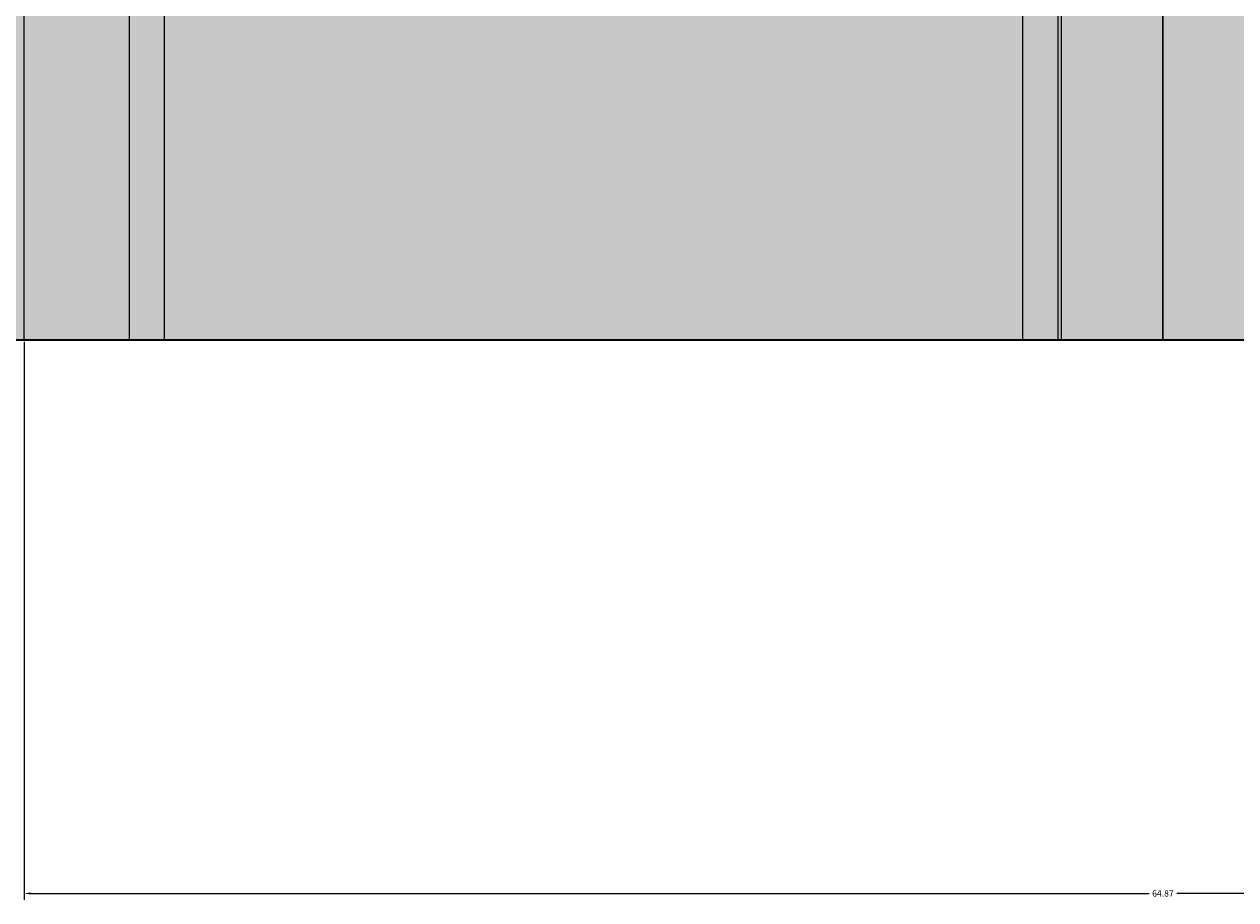
# Model space of a CAD drawing. Units: feet. Extents: x 2695 to 2912, y 795 to 1139.
# Tile 16 of 83: x 2774 to 2808, y 795 to 820. Entities that reach past the tile are written whole.
import ezdxf

# ---------------------------------------------------------------- set-up
doc = ezdxf.new("R2010")
doc.units = ezdxf.units.FT
for name, color, linetype, lineweight in [('A-ANNO-DIMS', 2, 'Continuous', 18), ('A-DOOR', 3, 'Continuous', 25), ('A-DOOR-PATT', 33, 'Continuous', 13), ('A-ELEV', 7, 'Continuous', 35), ('A-ELEV-PATT', 252, 'Continuous', 13)]:
    doc.layers.add(name, color=color, linetype=linetype, lineweight=lineweight)
doc.styles.get("Standard").update_dxf_attribs({"font": 'arial.ttf'})
doc.dimstyles.get("Standard").update_dxf_attribs({"dimtxt": 0.18, "dimasz": 0.18, "dimexe": 0.18, "dimexo": 0.0625, "dimgap": 0.09, "dimtad": 0, "dimtih": 1, "dimtoh": 1, "dimdec": 1, "dimzin": 0, "dimdsep": 46, "dimlunit": 3, "dimtxsty": 'Standard', "dimcen": 0.09, "dimadec": 0, "dimazin": 0, "dimtfac": 1, "dimtdec": 1, "dimtofl": 0, "dimtmove": 0, "dimatfit": 3, "dimfxl": 1, "dimtolj": 1, "dimtzin": 0, "dimarcsym": 0})

# ---------------------------------------------------------------- blocks, each defined once
blk = doc.blocks.new('*D5')
at = {"layer": 'A-ANNO-DIMS', "color": 0, "lineweight": -2, "transparency": 16777216}
for p, q in [((2773.503, 810.868), (2773.503, 794.976)), ((2838.377, 810.868), (2838.377, 794.976)), ((2773.683, 795.156), (2805.546, 795.156)), ((2838.197, 795.156), (2806.334, 795.156))]:
    blk.add_line(p, q, dxfattribs=at)
at = {"layer": 'A-ANNO-DIMS', "color": 0, "transparency": 16777216}
for points in [[(2773.683, 795.186), (2773.683, 795.126), (2773.503, 795.156)], [(2838.197, 795.186), (2838.197, 795.126), (2838.377, 795.156)]]:
    blk.add_solid(points, dxfattribs=at)
at = {"layer": 'Defpoints', "color": 0, "transparency": 16777216}
for p in [(2773.503, 810.931), (2838.377, 810.931), (2838.377, 795.156)]:
    blk.add_point(p, dxfattribs=at)
at = {"layer": 'A-ANNO-DIMS', "color": 0, "transparency": 16777216, "insert": (2805.94, 795.156), "char_height": 0.18, "attachment_point": 5}
blk.add_mtext('\\A1;64.87', dxfattribs=at)
blk = doc.blocks.new('*D13')
at = {"layer": 'A-ANNO-DIMS', "color": 0, "lineweight": -2, "transparency": 16777216}
for p, q in [((2758.214, 874.857), (2911.424, 874.857)), ((2911.244, 874.677), (2911.244, 843.076)), ((2911.244, 811.111), (2911.244, 842.712)), ((2890.699, 810.931), (2911.424, 810.931))]:
    blk.add_line(p, q, dxfattribs=at)
at = {"layer": 'A-ANNO-DIMS', "color": 0, "transparency": 16777216}
for points in [[(2911.214, 874.677), (2911.274, 874.677), (2911.244, 874.857)], [(2911.214, 811.111), (2911.274, 811.111), (2911.244, 810.931)]]:
    blk.add_solid(points, dxfattribs=at)
at = {"layer": 'Defpoints', "color": 0, "transparency": 16777216}
for p in [(2758.151, 874.857), (2911.244, 874.857), (2890.636, 810.931)]:
    blk.add_point(p, dxfattribs=at)
at = {"layer": 'A-ANNO-DIMS', "color": 0, "transparency": 16777216, "insert": (2911.244, 842.894), "char_height": 0.18, "attachment_point": 5}
blk.add_mtext('\\A1;63.93', dxfattribs=at)

msp = doc.modelspace()

# ---------------------------------------------------------------- hatches: boundary and pattern name
at = {"layer": 'A-DOOR-PATT'}
h = msp.add_hatch(color=256, dxfattribs=at)
h.set_gradient(color1=(211, 185, 150), color2=(211, 185, 150))
h.paths.add_polyline_path([(2805.9398, 905.5143), (2773.5029, 905.5143), (2773.5029, 810.9306), (2776.4999, 810.9306), (2776.4999, 902.5174), (2802.9429, 902.5174), (2802.9429, 810.9306), (2805.9398, 810.9306)])
h.paths.add_polyline_path([(2803.9681, 874.1057), (2805.0538, 874.1057), (2805.0538, 846.2857), (2803.9681, 846.2857)], flags=16)
h.paths.add_polyline_path([(2838.3767, 905.5143), (2805.9398, 905.5143), (2805.9398, 810.9306), (2808.9368, 810.9306), (2808.9368, 902.5174), (2835.3798, 902.5174), (2835.3798, 810.9306), (2838.3767, 810.9306)])
h = msp.add_hatch(color=256, dxfattribs=at)
h.set_gradient(color1=(211, 185, 150), color2=(211, 185, 150))
h.paths.add_polyline_path([(2777.5029, 901.5143), (2801.9398, 901.5143), (2801.9398, 810.9306), (2802.9429, 810.9306), (2802.9429, 902.5174), (2776.4999, 902.5174), (2776.4999, 810.9306), (2777.5029, 810.9306)])
h.paths.add_polyline_path([(2809.9398, 901.5143), (2834.3767, 901.5143), (2834.3767, 810.9306), (2835.3798, 810.9306), (2835.3798, 902.5174), (2808.9368, 902.5174), (2808.9368, 810.9306), (2809.9398, 810.9306)])
h = msp.add_hatch(color=256, dxfattribs=at)
h.set_gradient(color1=(173, 221, 247), color2=(173, 221, 247))
h.paths.add_polyline_path([(2801.9398, 901.5143), (2777.5029, 901.5143), (2777.5029, 810.9306), (2801.9398, 810.9306)])
h.paths.add_polyline_path([(2834.3767, 901.5143), (2809.9398, 901.5143), (2809.9398, 810.9306), (2834.3767, 810.9306)])
at = {"layer": 'A-ELEV-PATT'}
h = msp.add_hatch(color=256, dxfattribs=at)
h.set_gradient(color1=(147, 149, 152), color2=(147, 149, 152), tint=1)
h.paths.add_polyline_path([(2770.6361, 1118.4096), (2710.6361, 1118.4096), (2710.6361, 1062.9306), (2770.6361, 1062.9306)])
h.paths.add_polyline_path([(2890.6361, 1103.3378), (2770.6361, 1103.3378), (2770.6361, 1062.9306), (2890.6361, 1062.9306)])
h.paths.add_polyline_path([(2730.7081, 1048.1052), (2755.1125, 1048.1052), (2755.1125, 936.9306), (2770.6361, 936.9306), (2770.6361, 1050.3105), (2715.8852, 1050.3105), (2715.8852, 936.9306), (2730.7081, 936.9306)])
h.paths.add_polyline_path([(2890.6361, 1050.3105), (2770.6361, 1050.3105), (2770.6361, 971.9673), (2778.0341, 971.9673), (2778.0341, 1020.8235), (2843.575, 1020.8235), (2843.575, 971.9673), (2890.6361, 971.9673)])
h.paths.add_polyline_path([(2888.1882, 970.7156), (2843.575, 970.7156), (2843.575, 964.8267), (2888.1882, 964.8267)])
h.paths.add_polyline_path([(2888.1882, 964.1328), (2843.575, 964.1328), (2843.575, 956.614), (2888.1882, 956.614)])
h.paths.add_polyline_path([(2888.1882, 955.9202), (2843.575, 955.9202), (2843.575, 949.2892), (2888.1882, 949.2892)])
h.paths.add_polyline_path([(2888.1882, 948.5954), (2843.575, 948.5954), (2843.575, 941.3507), (2888.1882, 941.3507)])
h.paths.add_polyline_path([(2888.1882, 940.6569), (2843.575, 940.6569), (2843.575, 936.9306), (2888.1882, 936.9306)])
h.paths.add_polyline_path([(2890.6361, 970.7156), (2888.9368, 970.7156), (2888.9368, 964.8267), (2890.6361, 964.8267)])
h.paths.add_polyline_path([(2890.6361, 964.1328), (2888.9368, 964.1328), (2888.9368, 956.614), (2890.6361, 956.614)])
h.paths.add_polyline_path([(2890.6361, 955.9202), (2888.9368, 955.9202), (2888.9368, 949.2892), (2890.6361, 949.2892)])
h.paths.add_polyline_path([(2890.6361, 940.6569), (2888.9368, 940.6569), (2888.9368, 936.9306), (2890.6361, 936.9306)])
h.paths.add_polyline_path([(2890.6361, 948.5954), (2888.9368, 948.5954), (2888.9368, 941.3507), (2890.6361, 941.3507)])
h.paths.add_polyline_path([(2772.5216, 970.7156), (2770.6361, 970.7156), (2770.6361, 964.8267), (2772.5216, 964.8267)])
h.paths.add_polyline_path([(2772.5216, 964.1328), (2770.6361, 964.1328), (2770.6361, 956.614), (2772.5216, 956.614)])
h.paths.add_polyline_path([(2772.5216, 955.9202), (2770.6361, 955.9202), (2770.6361, 949.2892), (2772.5216, 949.2892)])
h.paths.add_polyline_path([(2772.5216, 948.5954), (2770.6361, 948.5954), (2770.6361, 941.3507), (2772.5216, 941.3507)])
h.paths.add_polyline_path([(2772.5216, 940.6569), (2770.6361, 940.6569), (2770.6361, 936.9306), (2772.5216, 936.9306)])
h.paths.add_polyline_path([(2778.0341, 940.6569), (2773.2702, 940.6569), (2773.2702, 936.9306), (2778.0341, 936.9306)])
h.paths.add_polyline_path([(2778.0341, 970.7156), (2773.2702, 970.7156), (2773.2702, 964.8267), (2778.0341, 964.8267)])
h.paths.add_polyline_path([(2778.0341, 964.1328), (2773.2702, 964.1328), (2773.2702, 956.614), (2778.0341, 956.614)])
h.paths.add_polyline_path([(2778.0341, 955.9202), (2773.2702, 955.9202), (2773.2702, 949.2892), (2778.0341, 949.2892)])
h.paths.add_polyline_path([(2778.0341, 948.5954), (2773.2702, 948.5954), (2773.2702, 941.3507), (2778.0341, 941.3507)])
h.paths.add_polyline_path([(2810.0407, 940.6569), (2780.0341, 940.6569), (2780.0341, 936.9306), (2810.0407, 936.9306)])
h.paths.add_polyline_path([(2890.6361, 924.3105), (2770.6361, 924.3105), (2770.6361, 810.9306), (2773.5029, 810.9306), (2773.5029, 905.5143), (2805.9398, 905.5143), (2838.3767, 905.5143), (2838.3767, 810.9306), (2890.6361, 810.9306)])

# ---------------------------------------------------------------- linework, layer by layer
at = {"layer": 'A-DOOR'}
for points in [[(2773.5029, 810.9306), (2773.5029, 905.5143), (2805.9398, 905.5143), (2805.9398, 810.9306)], [(2838.3767, 810.9306), (2838.3767, 905.5143), (2805.9398, 905.5143), (2805.9398, 810.9306)], [(2776.4999, 810.9306), (2776.4999, 902.5174), (2802.9429, 902.5174), (2802.9429, 810.9306)], [(2777.5029, 810.9306), (2777.5029, 901.5143), (2801.9398, 901.5143), (2801.9398, 810.9306)]]:
    msp.add_lwpolyline(points, dxfattribs=at)
for points in [[(2773.5029, 905.5143), (2838.3767, 905.5143), (2838.3767, 810.9306), (2773.5029, 810.9306)], [(2805.9398, 905.5143), (2805.9398, 905.5143), (2805.9398, 810.9306), (2805.9398, 810.9306)], [(2776.4999, 902.5174), (2803.0393, 902.5174), (2803.0393, 810.9306), (2776.4999, 810.9306)], [(2777.5029, 901.5143), (2801.9398, 901.5143), (2801.9398, 810.9306), (2777.5029, 810.9306)]]:
    msp.add_lwpolyline(points, close=True, dxfattribs=at)
at = {"layer": 'A-ELEV'}
for q in [(2890.6361, 810.9306), (2890.6361, 810.9306), (2895.4426, 810.9306)]:
    msp.add_line((2710.6361, 810.9306), q, dxfattribs=at)

# ---------------------------------------------------------------- dimensions: what is measured, and where the dimension line sits
at = {"layer": 'A-ANNO-DIMS'}
dim = msp.add_linear_dim(base=(2911.2444, 874.8571), p1=(2890.6361, 810.9306), p2=(2758.1515, 874.8571), angle=90, dimstyle='Standard', override={"dimdec": 2, "dimlfac": 1, "dimrnd": 0, "dimzin": 0, "dimdsep": 46, "dimlunit": 2}, dxfattribs=at)
dim.commit()
dim.dimension.update_dxf_attribs({"geometry": '*D13', "text_midpoint": (2911.2444, 842.8938)})
dim = msp.add_linear_dim(base=(2838.3767, 795.1556), p1=(2773.5029, 810.9306), p2=(2838.3767, 810.9306), dimstyle='Standard', override={"dimdec": 2, "dimlfac": 1, "dimrnd": 0, "dimzin": 0, "dimdsep": 46, "dimlunit": 2}, dxfattribs=at)
dim.commit()
dim.dimension.update_dxf_attribs({"geometry": '*D5', "text_midpoint": (2805.9398, 795.1556)})

doc.saveas('drawing.dxf')
